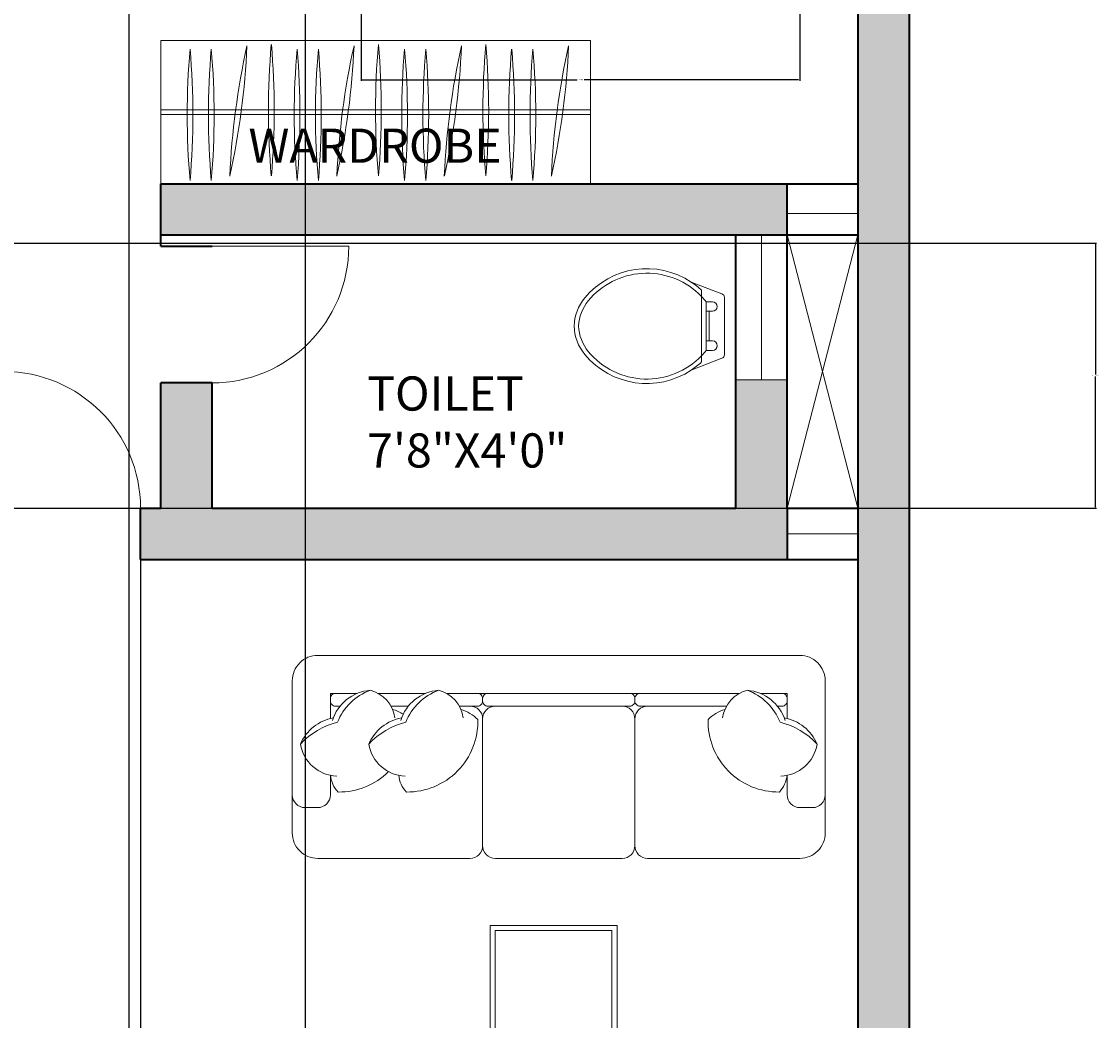
# Model space of a CAD drawing. Units: inches. Extents: x 37 to 706, y -568 to 110.
# Tile 23 of 24: x 517 to 706, y -233 to -57. Entities that reach past the tile are written whole.
import ezdxf

# ---------------------------------------------------------------- set-up
doc = ezdxf.new("R2010")
doc.units = ezdxf.units.IN
doc.header["$MEASUREMENT"] = 0
for name, color, linetype, lineweight in [('A-ANNO-DIMS', 2, 'Continuous', 18), ('A-ANNO-TEXT', 7, 'Continuous', 18), ('A-AREA-IDEN', 7, 'Continuous', 18), ('A-DOOR', 4, 'Continuous', 18), ('A-FLOR-CASE', 9, 'Continuous', 18), ('A-FLOR-FIXT', 9, 'Continuous', 18), ('A-FLOR-OPEN', 8, 'Continuous', 13), ('A-FURN', 8, 'Continuous', 13), ('A-GLAZ', 4, 'Continuous', 18), ('A-WALL', 7, 'Continuous', 35), ('A-WALL-PATT', 252, 'Continuous', 13)]:
    doc.layers.add(name, color=color, linetype=linetype, lineweight=lineweight)
doc.styles.get("Standard").update_dxf_attribs({"font": 'arial.ttf'})
doc.dimstyles.get("Standard").update_dxf_attribs({"dimtxt": 0.18, "dimasz": 0.18, "dimexe": 0.18, "dimexo": 0.0625, "dimgap": 0.09, "dimtad": 0, "dimtih": 1, "dimtoh": 1, "dimdec": 0, "dimzin": 0, "dimdsep": 46, "dimlunit": 3, "dimtxsty": 'Standard', "dimcen": 0.09, "dimadec": 0, "dimazin": 0, "dimtfac": 1, "dimtdec": 0, "dimtofl": 0, "dimtmove": 0, "dimatfit": 3, "dimfxl": 1, "dimtolj": 1, "dimtzin": 0, "dimarcsym": 0})

# ---------------------------------------------------------------- blocks, each defined once
blk = doc.blocks.new('WARDROBE-DOUBLE')
for p, q in [((75.49, 25.16), (0, 25.16)), ((0, 25.16), (0, 0)), ((75.49, 25.16), (75.49, 0)), ((75.49, 13), (0, 13)), ((75.49, 12.16), (0, 12.16)), ((75.49, 0), (0, 0))]:
    blk.add_line(p, q)
for centre, start, end in [((137.01, 12.08), 175.0028, 184.9972), ((-126.78, 12.08), 355.0028, 4.9972), ((140.74, 12.08), 175.0028, 184.9972), ((-123.05, 12.08), 355.0028, 4.9972), ((-117.16, 29.99), 347.508, 357.5023), ((144.38, -4.42), 167.508, 177.5023), ((151.29, 12.89), 175.0028, 184.9972), ((-112.5, 12.89), 355.0028, 4.9972), ((155.82, 12.08), 175.0028, 184.9972), ((-107.97, 12.08), 355.0028, 4.9972), ((159.55, 12.08), 175.0028, 184.9972), ((-104.24, 12.08), 355.0028, 4.9972), ((-98.35, 29.99), 347.508, 357.5023), ((163.19, -4.42), 167.508, 177.5023), ((170.1, 12.89), 175.0028, 184.9972), ((-93.69, 12.89), 355.0028, 4.9972), ((174.7, 12.08), 175.0028, 184.9972), ((-89.09, 12.08), 355.0028, 4.9972), ((178.43, 12.08), 175.0028, 184.9972), ((-85.36, 12.08), 355.0028, 4.9972), ((182.06, -4.42), 167.508, 177.5023), ((-79.47, 29.99), 347.508, 357.5023), ((188.97, 12.89), 175.0028, 184.9972), ((-74.82, 12.89), 355.0028, 4.9972), ((193.51, 12.08), 175.0028, 184.9972), ((-70.28, 12.08), 355.0028, 4.9972), ((197.24, 12.08), 175.0028, 184.9972), ((-66.55, 12.08), 355.0028, 4.9972), ((200.87, -4.42), 167.508, 177.5023), ((-60.66, 29.99), 347.508, 357.5023)]:
    blk.add_arc(centre, 132.4, start, end)
blk = doc.blocks.new('WC-PLAN')
for p, q in [((22.41, 16.39), (22.41, 15.28)), ((22.41, 15.28), (22.41, 10.09)), ((22.41, 4.89), (22.41, 10.09)), ((22.41, 4.89), (22.41, 3.79))]:
    blk.add_line(p, q)
for points in [[(20.6, 17.82, 0.383919), (1.9, 15.05, 0.163732), (0, 10.09, 0.359733)], [(21.87, 15.81, 0.431639), (2.51, 14.55, 0.162618), (0.79, 10.09, 0.470877)], [(22.41, 16.39, 0.040937), (20.6, 17.82, 0.163732)], [(26.41, 10.09), (26.41, 15.13, 0.31031), (25.98, 15.75), (20.6, 17.82, 0.209071)], [(22.41, 15.28, 0.014165), (21.87, 15.81, 0.162618)], [(23.21, 14.37, 0.022712), (22.41, 15.28, 0.162618)], [(23.21, 10.09), (23.21, 14.37, 0.022712)], [(23.21, 14.37), (24.32, 14.37, -1), (24.32, 12.69), (23.74, 12.69)], [(20.6, 2.36, -0.383919), (1.9, 5.12, -0.163732), (0, 10.09, -0.359733)], [(22.41, 4.89, -0.448546), (2.51, 5.63, -0.162618), (0.79, 10.09, -0.470877)], [(26.41, 10.09), (26.41, 5.05, -0.31031), (25.98, 4.43), (20.6, 2.36, -0.209071)], [(23.21, 10.09), (23.21, 5.8, -0.476108)], [(23.21, 5.8, -0.022712), (22.41, 4.89, -0.162618)], [(23.21, 5.8), (24.32, 5.8, 1), (24.32, 7.49), (23.74, 7.49)], [(22.41, 3.79, -0.040937), (20.6, 2.36, -0.163732)]]:
    blk.add_lwpolyline(points, format="xyb")
for points in [[(23.74, 12.69), (23.21, 12.69)], [(23.74, 7.49), (23.74, 12.69)], [(23.74, 7.49), (23.21, 7.49)]]:
    blk.add_lwpolyline(points)
blk = doc.blocks.new('COFFEE-TABLE-SQUARE')
at = {"ltscale": 0.03}
blk.add_lwpolyline([(22.29, 0), (0, 0), (0, 22.29), (22.29, 22.29)], close=True, dxfattribs=at)
blk.add_lwpolyline([(0.89, 0.89), (21.4, 0.89), (21.4, 21.4), (0.89, 21.4)], close=True)
blk = doc.blocks.new('DOOR-SWING-24')
blk.add_line((0, 0), (0, 24))
blk.add_arc((0, 0), 24, 0, 90)
blk = doc.blocks.new('*D24')
at = {"layer": 'A-ANNO-DIMS', "color": 0, "lineweight": -2, "transparency": 16777216}
for p, q in [((576.73, -53.97), (576.73, -67.67)), ((653.75, -53.97), (653.75, -67.67)), ((576.91, -67.49), (614.6, -67.49)), ((653.57, -67.49), (615.88, -67.49))]:
    blk.add_line(p, q, dxfattribs=at)
at = {"layer": 'A-ANNO-DIMS', "color": 0, "transparency": 16777216}
for points in [[(576.91, -67.46), (576.91, -67.52), (576.73, -67.49)], [(653.57, -67.46), (653.57, -67.52), (653.75, -67.49)]]:
    blk.add_solid(points, dxfattribs=at)
at = {"layer": 'Defpoints', "color": 0, "transparency": 16777216}
for p in [(576.73, -53.9), (653.75, -53.9), (653.75, -67.49)]:
    blk.add_point(p, dxfattribs=at)
at = {"layer": 'A-ANNO-DIMS', "color": 0, "transparency": 16777216, "insert": (615.24, -67.49), "char_height": 0.18, "attachment_point": 5}
blk.add_mtext('\\A1;6\'-5" TYP.', dxfattribs=at)
blk = doc.blocks.new('*D52')
at = {"layer": 'A-ANNO-DIMS', "color": 0, "lineweight": -2, "transparency": 16777216}
for p, q in [((535.96, -303.65), (535.96, 84.22)), ((536.14, 84.04), (551.13, 84.04)), ((566.78, 84.04), (551.79, 84.04)), ((566.96, -303.65), (566.96, 84.22))]:
    blk.add_line(p, q, dxfattribs=at)
at = {"layer": 'A-ANNO-DIMS', "color": 0, "transparency": 16777216}
for points in [[(536.14, 84.07), (536.14, 84.01), (535.96, 84.04)], [(566.78, 84.07), (566.78, 84.01), (566.96, 84.04)]]:
    blk.add_solid(points, dxfattribs=at)
at = {"layer": 'Defpoints', "color": 0, "transparency": 16777216}
for p in [(566.96, 84.04), (535.96, -303.71), (566.96, -303.71)]:
    blk.add_point(p, dxfattribs=at)
at = {"layer": 'A-ANNO-DIMS', "color": 0, "transparency": 16777216, "insert": (551.46, 84.04), "char_height": 0.18, "attachment_point": 5}
blk.add_mtext('\\A1;2\'-7"', dxfattribs=at)
blk = doc.blocks.new('*D53')
at = {"layer": 'A-ANNO-DIMS', "color": 0, "lineweight": -2, "transparency": 16777216}
for p, q in [((511.96, -151.77), (511.96, -567.64)), ((537.96, -151.77), (537.96, -567.64)), ((512.14, -567.46), (524.63, -567.46)), ((537.78, -567.46), (525.29, -567.46))]:
    blk.add_line(p, q, dxfattribs=at)
at = {"layer": 'A-ANNO-DIMS', "color": 0, "transparency": 16777216}
for points in [[(512.14, -567.43), (512.14, -567.49), (511.96, -567.46)], [(537.78, -567.43), (537.78, -567.49), (537.96, -567.46)]]:
    blk.add_solid(points, dxfattribs=at)
at = {"layer": 'Defpoints', "color": 0, "transparency": 16777216}
for p in [(511.96, -151.71), (537.96, -151.71), (537.96, -567.46)]:
    blk.add_point(p, dxfattribs=at)
at = {"layer": 'A-ANNO-DIMS', "color": 0, "transparency": 16777216, "insert": (524.96, -567.46), "char_height": 0.18, "attachment_point": 5}
blk.add_mtext('\\A1;2\'-2"', dxfattribs=at)
blk = doc.blocks.new('*D58')
at = {"layer": 'A-ANNO-DIMS', "color": 0, "lineweight": -2, "transparency": 16777216}
for p, q in [((405.88, -96.15), (705.89, -96.15)), ((705.71, -96.33), (705.71, -119.25)), ((705.71, -142.53), (705.71, -119.61)), ((403.02, -142.71), (705.89, -142.71))]:
    blk.add_line(p, q, dxfattribs=at)
at = {"layer": 'A-ANNO-DIMS', "color": 0, "transparency": 16777216}
for points in [[(705.68, -96.33), (705.74, -96.33), (705.71, -96.15)], [(705.68, -142.53), (705.74, -142.53), (705.71, -142.71)]]:
    blk.add_solid(points, dxfattribs=at)
at = {"layer": 'Defpoints', "color": 0, "transparency": 16777216}
for p in [(405.82, -96.15), (705.71, -96.15), (402.96, -142.71)]:
    blk.add_point(p, dxfattribs=at)
at = {"layer": 'A-ANNO-DIMS', "color": 0, "transparency": 16777216, "insert": (705.71, -119.43), "char_height": 0.18, "attachment_point": 5}
blk.add_mtext('\\A1;3\'-10 1/2"', dxfattribs=at)

msp = doc.modelspace()

# ---------------------------------------------------------------- hatches: boundary and pattern name
at = {"layer": 'A-WALL-PATT'}
h = msp.add_hatch(color=256, dxfattribs=at)
h.dxf.hatch_style = 1
h.paths.add_polyline_path([(220.96, -351.71), (211.96, -351.71), (211.96, -513.71), (254.96, -513.71), (254.96, -504.71), (220.96, -504.71)], flags=17)
h.paths.add_polyline_path([(220.96, -294.71), (211.96, -294.71), (211.96, -303.71), (220.96, -303.71)], flags=17)
h.paths.add_polyline_path([(175.96, -294.71), (155.87, -294.71), (155.87, -303.71), (155.96, -303.71), (175.96, -303.71)], flags=17)
h.paths.add_polyline_path([(220.96, -16.71), (211.96, -16.71), (211.96, -142.71), (220.96, -142.71)], flags=17)
h.paths.add_polyline_path([(357.96, 51.29), (78.96, 51.29), (78.96, -513.71), (87.96, -513.71), (87.96, -303.71), (95.87, -303.71), (95.87, -294.71), (87.96, -294.71), (87.96, -142.71), (187.96, -142.71), (187.96, -133.71), (87.96, -133.71), (87.96, -25.71), (106.96, -25.71), (106.96, -16.71), (87.96, -16.71), (87.96, 42.29), (348.96, 42.29), (348.96, 17.13), (348.96, -133.71), (246.96, -133.71), (246.96, -142.71), (348.96, -142.71), (348.96, -294.71), (251.96, -294.71), (251.96, -303.71), (348.96, -303.71), (348.96, -351.71), (260.96, -351.71), (260.96, -329.71), (251.96, -329.71), (251.96, -360.71), (327.45, -360.71), (348.96, -360.71), (348.96, -504.71), (314.96, -504.71), (314.96, -513.71), (357.96, -513.71)])
h.paths.add_polyline_path([(416.96, -303.71), (402.96, -303.71), (402.96, -151.71), (478.96, -151.71), (478.96, -142.71), (402.96, -142.71), (402.96, -22.71), (409.96, -22.71), (409.96, -13.71), (402.96, -13.71), (402.96, 42.29), (663.96, 42.29), (663.96, -303.71), (566.96, -303.71), (566.96, -312.71), (663.96, -312.71), (663.96, -360.71), (575.96, -360.71), (575.96, -338.71), (566.96, -338.71), (566.96, -360.71), (566.96, -369.71), (642.45, -369.71), (663.96, -369.71), (663.96, -513.71), (629.96, -513.71), (629.96, -522.71), (672.96, -522.71), (672.96, 51.29), (393.96, 51.29), (393.96, -522.71), (402.96, -522.71), (402.96, -312.71), (416.96, -312.71)])
h.paths.add_polyline_path([(490.96, -303.71), (476.96, -303.71), (476.96, -312.71), (490.96, -312.71)], flags=17)
h.paths.add_polyline_path([(535.96, -303.71), (526.96, -303.71), (526.96, -312.71), (535.96, -312.71)], flags=17)
h.paths.add_polyline_path([(535.96, -369.71), (526.96, -369.71), (526.96, -522.71), (569.96, -522.71), (569.96, -513.71), (535.96, -513.71)], flags=17)
h.paths.add_polyline_path([(511.96, -13.71), (502.96, -13.71), (502.96, -151.71), (511.96, -151.71)], flags=17)
h.paths.add_polyline_path([(651.54, -142.71), (651.54, -120.18), (642.54, -120.18), (642.54, -142.71), (550.54, -142.71), (550.54, -120.71), (541.54, -120.71), (541.54, -142.71), (537.96, -142.71), (537.96, -151.71), (651.54, -151.71)], flags=17)
h.paths.add_polyline_path([(651.54, -85.71), (541.54, -85.71), (541.54, -94.71), (651.54, -94.71)], flags=17)
h.paths.add_polyline_path([(476.96, -13.71), (469.96, -13.71), (469.96, -22.71), (476.96, -22.71)], flags=17)
h.paths.add_polyline_path([(185.96, -16.71), (166.96, -16.71), (166.96, -25.71), (185.96, -25.71)], flags=17)
h.paths.add_polyline_path([(168.91, -414.72), (214.62, -414.72), (214.62, -392.33), (168.91, -392.33)], flags=25)

# ---------------------------------------------------------------- linework, layer by layer
at = {"layer": 'A-FLOR-OPEN'}
for p, q in [((651.54, -94.71), (663.96, -142.71)), ((651.54, -142.71), (663.96, -94.71))]:
    msp.add_line(p, q, dxfattribs=at)
at = {"layer": 'A-FURN', "ltscale": 0.03}
msp.add_lwpolyline([(658.24, -199.78, -0.414214), (653.78, -204.24), (627.03, -204.24, -0.414214), (624.8, -202.01, -0.414214), (622.57, -204.24), (600.29, -204.24, -0.414214), (598.06, -202.01, -0.414214), (595.83, -204.24), (569.08, -204.24, -0.414214), (564.62, -199.78), (564.62, -173.03, -0.414214), (569.08, -168.58), (653.78, -168.58, -0.414214), (658.24, -173.03)], format="xyb", close=True, dxfattribs=at)
at = {"layer": 'A-FURN'}
for points in [[(566.04, -184.16, -0.14773), (572.56, -180.33, -0.213343), (578.3, -174.71, -0.178662)], [(576, -175.26), (571.31, -175.26), (571.31, -179.64, -0.414214)], [(573.01, -177.49), (572.2, -177.49, -0.414214), (571.31, -176.6), (571.31, -176.15, -0.414214), (572.2, -175.26)], [(571.66, -180.02, -0.306663), (578.3, -174.71, -0.30633), (582.65, -179.56, 0.872847)], [(572.2, -175.26), (576, -175.26, -0.414214)], [(578.05, -184.16, -0.14773), (584.56, -180.33, -0.213343), (590.31, -174.71, -0.178662)], [(579.71, -175.26), (588.01, -175.26, -0.414214)], [(583.66, -180.02, -0.306663), (590.31, -174.71, -0.30633), (594.65, -179.56, 0.872847)], [(591.71, -175.26), (597.17, -175.26, -0.414214), (598.06, -176.15), (598.06, -176.6, -0.414214), (597.17, -177.49), (593.96, -177.49, -0.414214)], [(643.15, -175.26), (625.69, -175.26, 0.414214), (624.8, -176.15), (624.8, -176.6, 0.414214), (625.69, -177.49), (640.91, -177.49, 0.414214)], [(651.2, -180.02, 0.306663), (644.56, -174.71, 0.30633), (640.21, -179.56, -0.872847)], [(656.82, -184.16, 0.14773), (650.3, -180.33, 0.213343), (644.56, -174.71, 0.178662)], [(650.66, -175.26), (646.86, -175.26, 0.414214)], [(649.85, -177.49), (650.66, -177.49, 0.414214), (651.55, -176.6), (651.55, -176.15, 0.414214), (650.66, -175.26)], [(585.02, -177.49), (581.95, -177.49, -0.414214)], [(595.83, -177.49, -0.414214), (598.06, -179.72), (598.06, -202.01, -0.414214)], [(600.29, -177.49, 0.414214), (598.06, -179.72)], [(622.57, -177.49, -0.414214), (624.8, -179.72)], [(627.03, -177.49, 0.414214), (624.8, -179.72), (624.8, -202.01, 0.414214)], [(572.43, -189.78, -0.356772), (566.04, -184.16, -0.249542), (571.83, -179.53, 9.61688)], [(584.44, -189.78, -0.356772), (578.05, -184.16, -0.249542), (583.84, -179.53, 9.61688)], [(584.1, -178.93, 0.071865), (582.23, -178.06, -7.115464)], [(583.31, -189.64, 0.165541), (584.69, -192.58, 0.425989), (597.21, -179.82, 0.121523), (594.24, -178.06, -7.115464)], [(651.55, -189.64, -0.165541), (650.18, -192.58, -0.425989), (637.66, -179.82, -0.121523), (640.63, -178.06, 7.115464)], [(650.43, -189.78, 0.356772), (656.82, -184.16, 0.249542), (651.03, -179.53, -9.61688)], [(571.31, -189.64, 0.165541), (572.68, -192.58, 0.200231), (581.53, -189, 0.121523)], [(571.31, -189.64), (571.31, -193.09, -0.414214), (569.08, -195.32), (566.85, -195.32, -0.414214), (564.62, -193.09)], [(658.24, -193.09, -0.414214), (656.01, -195.32), (653.78, -195.32, -0.414214), (651.55, -193.09), (651.55, -189.64)]]:
    msp.add_lwpolyline(points, format="xyb", dxfattribs=at)
for points in [[(588.01, -175.26), (579.71, -175.26)], [(643.15, -175.26), (591.71, -175.26)], [(651.55, -179.64), (651.55, -175.26), (646.86, -175.26)]]:
    msp.add_lwpolyline(points, dxfattribs=at)
msp.add_lwpolyline([(598.95, -175.26), (623.91, -175.26, -0.414214), (624.8, -176.15), (624.8, -176.6, -0.414214), (623.91, -177.49), (598.95, -177.49, -0.414214), (598.06, -176.6), (598.06, -176.15, -0.414214)], format="xyb", close=True, dxfattribs=at)
at = {"layer": 'A-GLAZ'}
for p, q in [((651.54, -90.97), (663.96, -90.97)), ((647.04, -120.18), (647.04, -94.71)), ((651.54, -120.18), (642.54, -120.18)), ((651.54, -147.21), (663.96, -147.21))]:
    msp.add_line(p, q, dxfattribs=at)
at = {"layer": 'A-WALL'}
for p, q in [((672.96, 51.29), (672.96, -522.71)), ((663.96, 42.29), (663.96, -303.71)), ((541.54, -85.71), (663.96, -85.71)), ((541.54, -96.71), (541.54, -85.71)), ((651.54, -142.71), (651.54, -85.71)), ((541.54, -94.71), (663.96, -94.71)), ((642.54, -142.71), (642.54, -94.71)), ((541.54, -96.71), (550.54, -96.71)), ((541.54, -142.71), (541.54, -120.71)), ((550.54, -120.71), (541.54, -120.71)), ((550.54, -142.71), (550.54, -120.71)), ((537.96, -151.71), (537.96, -142.71)), ((537.96, -142.71), (541.54, -142.71)), ((550.54, -142.71), (642.54, -142.71)), ((651.54, -142.71), (651.54, -151.71)), ((651.54, -142.71), (663.96, -142.71)), ((537.96, -151.71), (663.96, -151.71))]:
    msp.add_line(p, q, dxfattribs=at)

# ---------------------------------------------------------------- block references
at = {"layer": 'A-DOOR', "rotation": 269.9999999999999}
msp.add_blockref('DOOR-SWING-24', (550.54, -96.71), dxfattribs=at)
at = {"layer": 'A-DOOR'}
msp.add_blockref('DOOR-SWING-24', (513.96, -142.71), dxfattribs=at)
at = {"layer": 'A-FLOR-CASE'}
msp.add_blockref('WARDROBE-DOUBLE', (541.54, -85.71), dxfattribs=at)
at = {"layer": 'A-FLOR-FIXT'}
msp.add_blockref('WC-PLAN', (614.11, -120.82), dxfattribs=at)
at = {"layer": 'A-FURN'}
msp.add_blockref('COFFEE-TABLE-SQUARE', (599.38, -238.33), dxfattribs=at)

# ---------------------------------------------------------------- texts
at = {"layer": 'A-ANNO-TEXT', "insert": (556.92, -76.04), "char_height": 6, "attachment_point": 1}
msp.add_mtext_dynamic_manual_height_columns('WARDROBE', width=0.234, gutter_width=1, heights=[0], dxfattribs=at)
at = {"layer": 'A-AREA-IDEN', "insert": (577.76, -119.57), "char_height": 6, "attachment_point": 1}
msp.add_mtext_dynamic_manual_height_columns('TOILET\\P7\'8"X4\'0"', width=0.522, gutter_width=1, heights=[0], dxfattribs=at)

# ---------------------------------------------------------------- dimensions: what is measured, and where the dimension line sits
at = {"layer": 'A-ANNO-DIMS'}
for base, p1, p2, picture, middle in [((566.96, 84.04), (535.96, -303.71), (566.96, -303.71), '*D52', (551.46, 84.04)), ((537.96, -567.46), (511.96, -151.71), (537.96, -151.71), '*D53', (524.96, -567.46))]:
    dim = msp.add_linear_dim(base=base, p1=p1, p2=p2, dimstyle='Standard', override={"dimdec": 1, "dimlfac": 1, "dimrnd": 0, "dimzin": 1, "dimdsep": 46, "dimlunit": 4, "dimfrac": 2}, dxfattribs=at)
    dim.commit()
    dim.dimension.update_dxf_attribs({"geometry": picture, "text_midpoint": middle})
dim = msp.add_linear_dim(base=(653.75, -67.49), p1=(576.73, -53.9), p2=(653.75, -53.9), text='<> TYP.', dimstyle='Standard', override={"dimdec": 1, "dimlfac": 1, "dimrnd": 0, "dimzin": 1, "dimdsep": 46, "dimlunit": 4, "dimfrac": 2}, dxfattribs=at)
dim.commit()
dim.dimension.update_dxf_attribs({"geometry": '*D24', "text_midpoint": (615.24, -67.49)})
dim = msp.add_linear_dim(base=(705.71, -96.15), p1=(402.96, -142.71), p2=(405.82, -96.15), angle=90, dimstyle='Standard', override={"dimdec": 1, "dimlfac": 1, "dimrnd": 0, "dimzin": 1, "dimdsep": 46, "dimlunit": 4, "dimfrac": 2}, dxfattribs=at)
dim.commit()
dim.dimension.update_dxf_attribs({"geometry": '*D58', "text_midpoint": (705.71, -119.43)})

doc.saveas('drawing.dxf')
